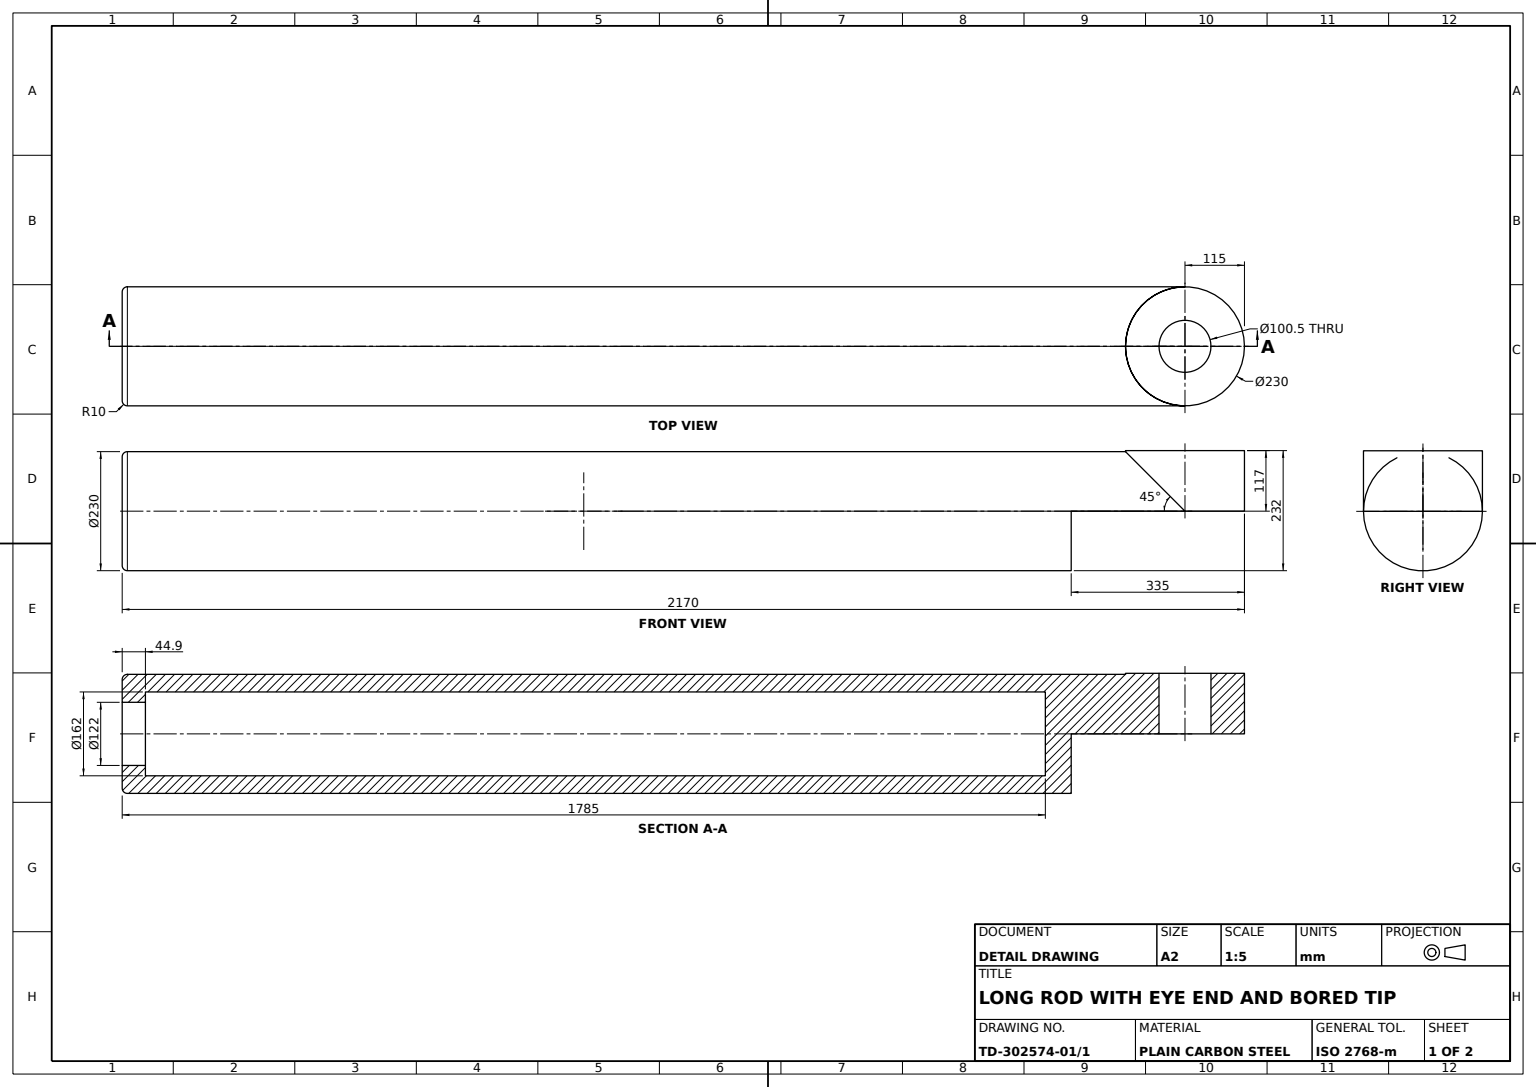
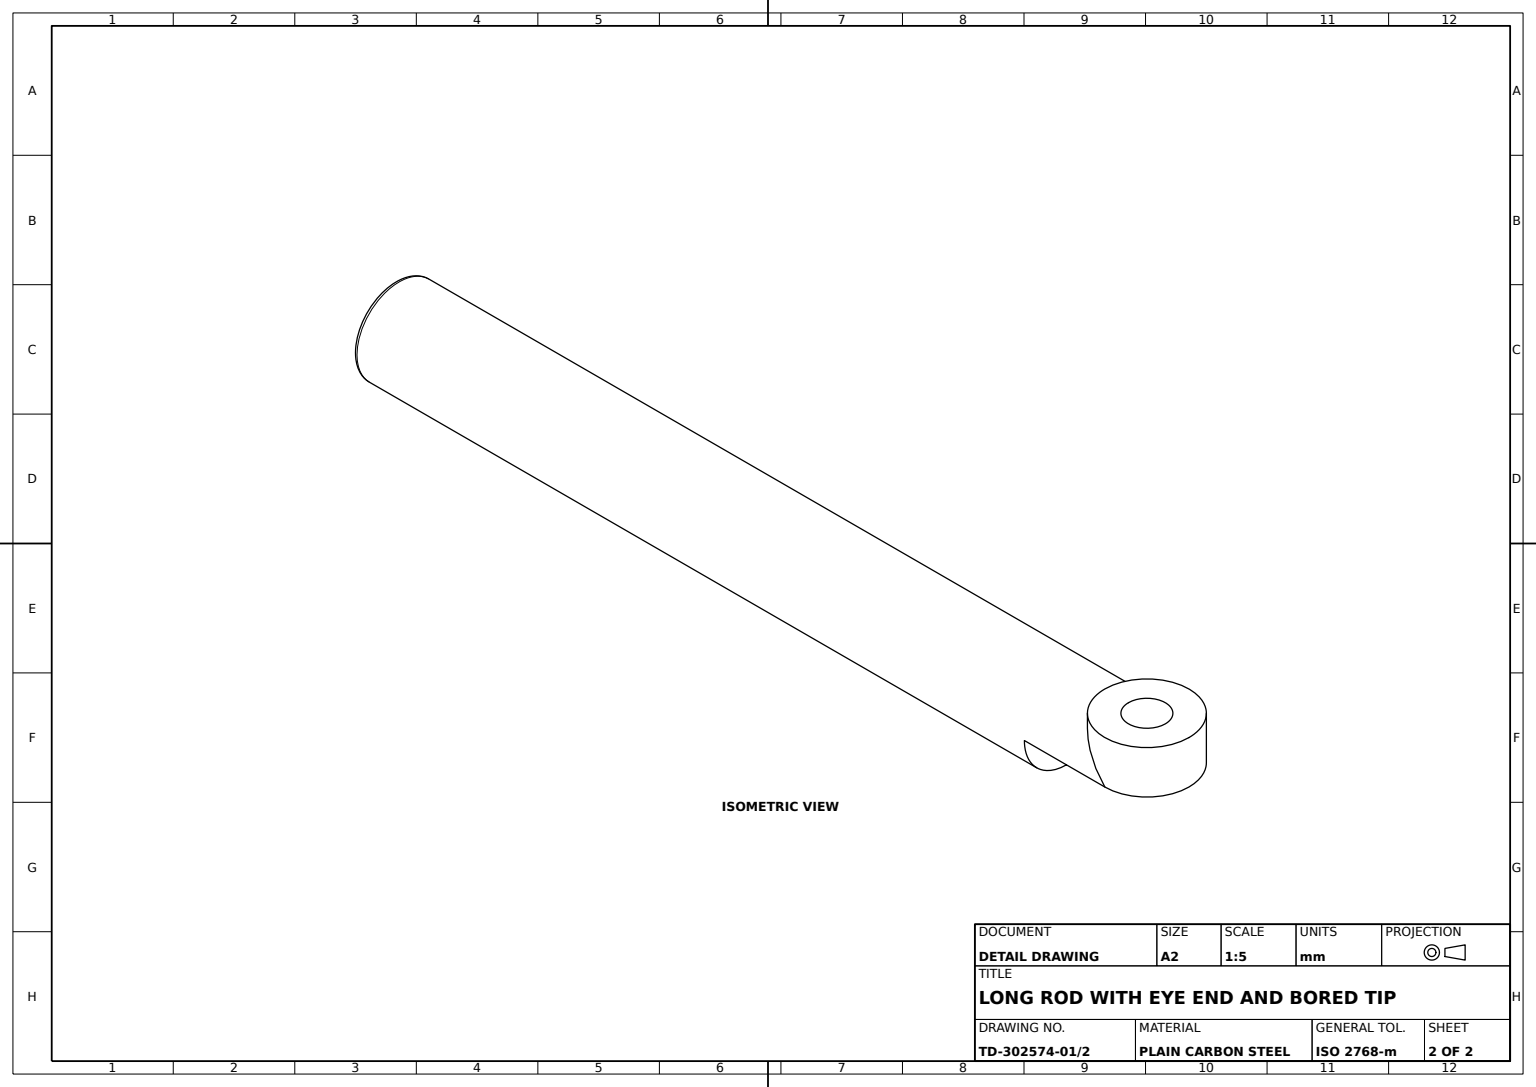
from build123d import *

# Parameters (mm, degrees)
BARREL_PROFILE_SKETCH_R  = 115
BARREL_BODY_230_DEPTH    = 1100
EYE_PIN_HOLE_SKETCH_R    = 50.25
EYE_PIN_HOLE_100_5_DEPTH = 1100
EYE_FLATS_SKETCH_W       = 230
EYE_FLATS_SKETCH_H       = 365
EYE_FLATS_CUT_DEPTH      = 2200
EYE_START                = -117
EYE_BOSS_SKETCH_R        = 115
EYE_BOSS_SKETCH_R_2      = 50.25
EYE_BOSS_EXTRUDE_DEPTH   = 117
EDGE_FILLET_R10_R        = 10


with BuildPart() as part:
    # Barrel Profile Sketch → Barrel Body Ø230 (new, symmetric)
    with BuildSketch(Plane.XY):
        Circle(BARREL_PROFILE_SKETCH_R)
    extrude(amount=BARREL_BODY_230_DEPTH, both=True)

    # Eye Pin Hole Sketch → Eye Pin Hole Ø100.5 (cut, symmetric)
    with BuildSketch(Plane(origin=(0, 0, 0), x_dir=(1, 0, 0), z_dir=(0, 1, 0))):
        with Locations(Location((0, 955, 0), (0, 0, 270))):
            Circle(EYE_PIN_HOLE_SKETCH_R)
    extrude(amount=EYE_PIN_HOLE_100_5_DEPTH, both=True, mode=Mode.SUBTRACT)

    # Eye Flats Sketch → Eye Flats Cut (cut)
    with BuildSketch(Plane(origin=(0, 0, 0), x_dir=(1, 0, 0), z_dir=(0, 1, 0))):
        with Locations((0, 917.5)):
            Rectangle(EYE_FLATS_SKETCH_W, EYE_FLATS_SKETCH_H)
    extrude(amount=-EYE_FLATS_CUT_DEPTH, mode=Mode.SUBTRACT)

    # Eye Transition Sketch → Eye Transition Revolve Cut (revolve, cut)
    with BuildSketch(Plane.XZ):
        with BuildLine():
            Line((-115, -955), (-196.346531204, -955))
            Line((-196.346531204, -955), (-196.346531204, -1191.859792513))
            Line((-196.346531204, -1191.859792513), (0, -1191.859792513))
            Line((0, -1191.859792513), (0, -1070))
            ThreePointArc((0, -1070), (-81.317279836, -1036.317279836), (-115, -955))
        make_face()
    revolve(axis=Axis((0, 0, -1191.859792513), (0, 0, 1)), mode=Mode.SUBTRACT)

    # End Bore Sketch → End Bore Revolve Cut (revolve, cut)
    with BuildSketch(Plane(origin=(0, 0, 0), x_dir=(1, 0, 0), z_dir=(0, 1, 0))):
        Polygon((0, -1100), (61, -1100), (61, -1055.102870795), (81, -1055.102870795), (81, 685), (0, 685), align=None)
    revolve(axis=Axis((0, 0, 1100), (0, 0, -1)), mode=Mode.SUBTRACT)

    # Eye Boss Sketch → Eye Boss Extrude (add)
    with BuildSketch(Plane.XZ.offset(EYE_START)):
        with Locations(Location((0, -955, 0), (0, 0, 270))):
            Circle(EYE_BOSS_SKETCH_R)
        with Locations(Location((0, -955, 0), (0, 0, 90))):
            Circle(EYE_BOSS_SKETCH_R_2, mode=Mode.SUBTRACT)
    extrude(amount=EYE_BOSS_EXTRUDE_DEPTH)

    # Edge Fillet R10
    edge_fillet_r10_edges = [part.edges().sort_by_distance(p)[0] for p in [
        (-115, 0, 1100),
    ]]
    fillet(edge_fillet_r10_edges, radius=EDGE_FILLET_R10_R)


solid = part.part
